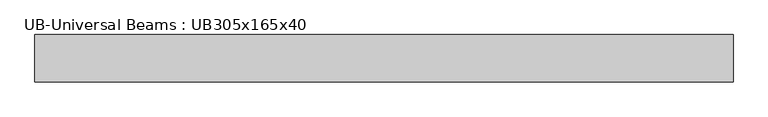
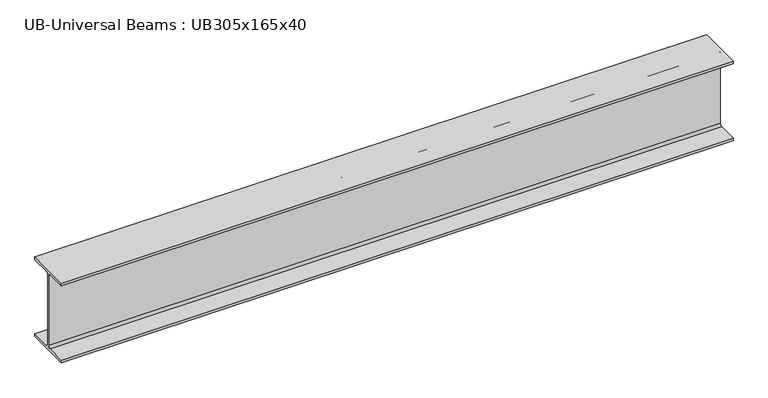
"""IFC4 building model written with IfcOpenShell, lengths in millimetres: beam geometry, UB-Universal Beams : UB305x165x40."""

from ifc_helpers import new_model, si_unit, point, frame, frame_2d, origin, place, context, project, spatial, polyline, circle_curve, trimmed, segment, composite_curve, outline, extrude, source, transform, mapped, element, save


def ub_universal_beams_ub305x165x40_1f6689ec(model_context):
    return source(origin(), model_context, "Body", "SweptSolid", [
        extrude(outline(composite_curve([segment(polyline([(82.5, -141.5), (82.5, -151.7), (-82.5, -151.7), (-82.5, -141.5), (-11.9, -141.5)]), True, "CONTINUOUS"), segment(trimmed(circle_curve(frame_2d((-11.9, -132.6)), 8.9), [point((-11.9, -141.5))], [point((-3.0, -132.6))], True, "CARTESIAN"), True, "CONTINUOUS"), segment(polyline([(-3.0, -132.6), (-3.0, 132.6)]), True, "CONTINUOUS"), segment(trimmed(circle_curve(frame_2d((-11.9, 132.6)), 8.9), [point((-3.0, 132.6))], [point((-11.9, 141.5))], True, "CARTESIAN"), True, "CONTINUOUS"), segment(polyline([(-11.9, 141.5), (-82.5, 141.5), (-82.5, 151.7), (82.5, 151.7), (82.5, 141.5), (11.9, 141.5)]), True, "CONTINUOUS"), segment(trimmed(circle_curve(frame_2d((11.9, 132.6)), 8.9), [point((11.9, 141.5))], [point((3.0, 132.6))], True, "CARTESIAN"), True, "CONTINUOUS"), segment(polyline([(3.0, 132.6), (3.0, -132.6)]), True, "CONTINUOUS"), segment(trimmed(circle_curve(frame_2d((11.9, -132.6)), 8.9), [point((3.0, -132.6))], [point((11.9, -141.5))], True, "CARTESIAN"), True, "CONTINUOUS"), segment(polyline([(11.9, -141.5), (82.5, -141.5)]), True, "CONTINUOUS")], self_intersect=False)), frame((-1165.85, 0.0, 0.0), z_axis=(1.0, 0.0, 0.0), x_axis=(0.0, 1.0, 0.0)), (0.0, 0.0, 1.0), 2422.0),
    ])


if __name__ == "__main__":
    model = new_model("IFC4")
    model_context = context("Model", 3, world=origin())
    ifc_project = project(units=[si_unit("LENGTHUNIT", "METRE", prefix="MILLI")], contexts=[model_context])
    site = spatial("IfcSite", under=ifc_project)
    building = spatial("IfcBuilding", under=site)
    placement = place(None, origin())
    ub_universal_beams_ub305x165x40_shape = ub_universal_beams_ub305x165x40_1f6689ec(model_context)
    element("IfcBeam", 1, ObjectType="UB-Universal Beams : UB305x165x40", at=placement, inside=building, context=model_context, shape_type="MappedRepresentation", body=[
        mapped(ub_universal_beams_ub305x165x40_shape, transform((0.0, 0.0, 0.0), x_axis=(1.0, 0.0, 0.0), y_axis=(0.0, 1.0, 0.0), z_axis=(0.0, 0.0, 1.0))),
    ])
    save(model, "model.ifc")

# Revit data of these elements
# Type "UB-Universal Beams : UB305x165x40"
#   Section Name Key = "UB305X165X40"
#   Width = 16.5 cm
#   Web Thickness = 0.6 cm
#   Web Fillet = 0.89 cm
#   Warping Constant = 164000.0 cm⁶
#   Torsional Moment of Inertia = 14.70 cm⁴
#   Section Area = 51.3 cm²
#   Plastic Modulus weak axis = 142.0 cm³
#   Plastic Modulus strong axis = 623.0 cm³
#   Nominal Weight = 40.2999 kgf/m
#   Moment of Inertia weak axis = 764.00 cm⁴
#   Moment of Inertia strong axis = 8503.00 cm⁴
#   Height = 30.34 cm
#   Flange Thickness = 1.02 cm
#   Elastic Modulus weak axis = 92.6 cm³
#   Elastic Modulus strong axis = 560.0 cm³
#   Centroid Vertical = 15.17 cm
#   Centroid Horizontal = 8.25 cm
#   Bolt Spacing = 9.0 cm
#   Length [instance default] = 1500 mm
#   Structural Material [instance default] = Metal - Steel 43-275
#   Type Comments = ""
#   Assembly Code = ""
# Element 1 (IfcBeam, "UB-Universal Beams : UB305x165x40")
#   Materials on its faces: "Metal - Steel 43-275"
# Materials
#   "Metal - Steel 43-275": class "Metal", colour RGB 247 247 247, transparency 0, Cost = 0
